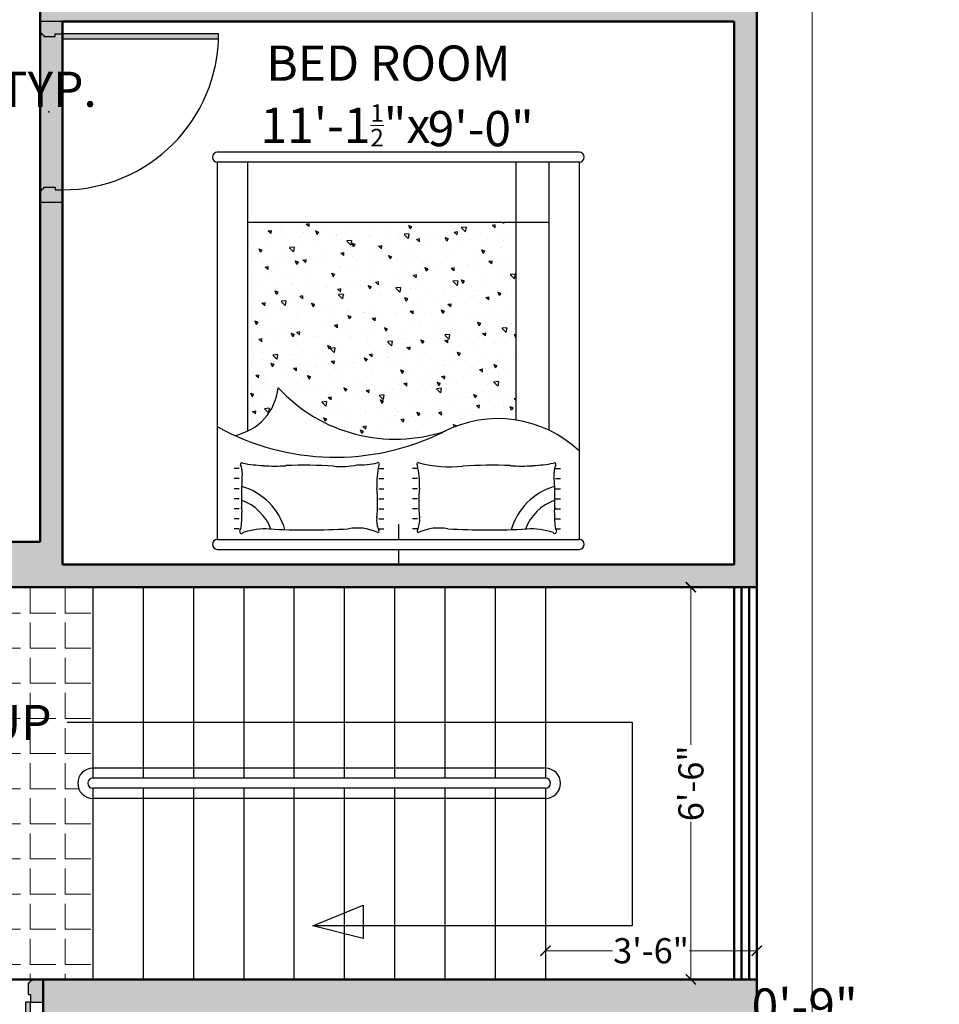
# Model space of a CAD drawing. Units: inches. Extents: x 4508 to 5907, y 877 to 1592.
# Tile 17 of 20: x 5383 to 5566, y 1298 to 1494. Entities that reach past the tile are written whole.
import ezdxf

# ---------------------------------------------------------------- set-up
doc = ezdxf.new("R2010")
doc.units = ezdxf.units.IN
doc.layers.get('DEFPOINTS').update_dxf_attribs({"color": 8})
for name, color, linetype, lineweight in [('A-ANNO-DIMS', 2, 'Continuous', 18), ('A-ANNO-TEXT', 7, 'Continuous', 25), ('A-DOOR', 4, 'Continuous', 25), ('A-FLOR-PATT', 252, 'Continuous', 13), ('A-FLOR-STRS', 5, 'Continuous', 25), ('A-FURN', 24, 'Continuous', 18), ('A-WALL', 7, 'Continuous', 50), ('A-WALL-PATT', 8, 'Continuous', 13)]:
    doc.layers.add(name, color=color, linetype=linetype, lineweight=lineweight)
doc.layers.add('doors & windows', color=30, linetype='Continuous')
doc.layers.add('furniture', color=24, linetype='Continuous')
doc.styles.get("Standard").update_dxf_attribs({"font": 'arial.ttf'})
doc.dimstyles.new('details', dxfattribs={"dimtxt": 5, "dimasz": 2, "dimexe": 2, "dimexo": 3, "dimgap": 1, "dimtad": 0, "dimdec": 1, "dimzin": 0, "dimdsep": 46, "dimlunit": 4, "dimtxsty": 'Standard', "dimblk": 'ARCHTICK', "dimcen": 3, "dimclrd": 256, "dimclre": 256, "dimclrt": 256, "dimadec": 0, "dimazin": 0, "dimtfac": 0.5, "dimtdec": 1, "dimtofl": 0, "dimtmove": 0, "dimatfit": 3, "dimldrblk": 'CLOSEDBLANK', "dimfxl": 2, "dimtolj": 1, "dimtzin": 0, "dimlwd": -1, "dimlwe": -1, "dimarcsym": 0})
doc.dimstyles.new('text', dxfattribs={"dimtxt": 7, "dimasz": 0, "dimexe": 3, "dimexo": 3, "dimgap": 0, "dimtad": 1, "dimtih": 1, "dimtoh": 1, "dimzin": 3, "dimdsep": 46, "dimlunit": 4, "dimtxsty": 'Standard', "dimblk": 'CLOSEDBLANK', "dimcen": 3, "dimse1": 1, "dimse2": 1, "dimsd1": 1, "dimsd2": 1, "dimclrd": 256, "dimclre": 256, "dimclrt": 256, "dimadec": 0, "dimazin": 0, "dimtfac": 0.5, "dimtofl": 0, "dimtmove": 0, "dimatfit": 3, "dimfxl": 3, "dimtolj": 1, "dimtzin": 0, "dimlwd": -1, "dimlwe": -1, "dimarcsym": 0})

# ---------------------------------------------------------------- blocks, each defined once
blk = doc.blocks.new('bed')
at = {"layer": 'furniture'}
h = blk.add_hatch(dxfattribs=at)
h.set_pattern_fill('AR-CONC', color=256, angle=-90, style=0)
h.set_pattern_definition([(320, (0, 2.38), (-0.6275, -7.1726), [0.75, -8.25]), (265, (0, 2.38), (7.5219, 1.3875), [0.6, -6.6]), (10.451, (-0.052, 1.782), (6.8944, -5.7851), [0.6374, -7.0114]), (316.184, (2, 2.38), (-1.6552, -10.6724), [1.125, -12.375]), (6.636, (1.862, 1.491), (9.7412, -9.3466), [0.9561, -10.5171]), (261.184, (2, 2.38), (9.7412, -9.3466), [0.9, -9.9]), (291, (1.5, 1.38), (-4.0262, -5.96907), [0.75, -8.25]), (236, (1.5, 1.38), (7.2515, -2.43315), [0.6, -6.6]), (341.451, (1.1645, 0.8826), (3.2253, -8.4022), [0.6374, -7.0114]), (307.5, (0, 2.38), (3.32894, -0.1216), [0, -6.52, 0, -6.7, 0, -6.625]), (277.5, (0, 2.38), (3.94412, -2.6307), [0, -3.82, 0, -6.37, 0, -2.525]), (237.5, (0, 4.61), (-0.22555, -5.33822), [0, -2.5, 0, -7.8, 0, -10.35]), (227.5, (0, 5.61), (1.00105, -5.83186), [0, -3.25, 0, -5.18, 0, -7.35])])
h.paths.add_polyline_path([(30.01, -68), (30.01, -26.5, 0.263043), (23.9, -35.15, 0.293424), (-9.18, -26.47, -0.156683), (-23.39, -28.72), (-23.39, -68)])
for p, q in [((0, -3), (0, 0)), ((36.01, -3), (-36.01, -3)), ((-36.01, -5), (-36.01, -80)), ((36.01, -5), (-36.01, -5)), ((0, -8), (0, -5)), ((36.01, -80), (36.01, -5)), ((-31.24, -7.07), (-32.24, -7.07)), ((-3.81, -7.07), (-2.81, -7.07)), ((3.89, -7.07), (2.89, -7.07)), ((31.63, -7.07), (32.63, -7.07)), ((-31.24, -9.07), (-32.24, -9.07)), ((-3.81, -9.07), (-2.81, -9.07)), ((3.89, -9.07), (2.89, -9.07)), ((31.63, -9.07), (32.63, -9.07)), ((-31.24, -11.07), (-32.24, -11.07)), ((-3.81, -11.07), (-2.81, -11.07)), ((3.89, -11.07), (2.89, -11.07)), ((31.63, -11.07), (32.63, -11.07)), ((-31.24, -13.07), (-32.24, -13.07)), ((-3.81, -13.07), (-2.81, -13.07)), ((3.89, -13.07), (2.89, -13.07)), ((31.63, -13.07), (32.63, -13.07)), ((-31.24, -15.07), (-32.24, -15.07)), ((-3.81, -15.07), (-2.81, -15.07)), ((3.89, -15.07), (2.89, -15.07)), ((31.63, -15.07), (32.63, -15.07)), ((-31.24, -17.07), (-32.24, -17.07)), ((-3.81, -17.07), (-2.81, -17.07)), ((3.89, -17.07), (2.89, -17.07)), ((31.63, -17.07), (32.63, -17.07)), ((-31.24, -19.07), (-32.24, -19.07)), ((-3.81, -19.07), (-2.81, -19.07)), ((3.89, -19.07), (2.89, -19.07)), ((31.63, -19.07), (32.63, -19.07)), ((-36.01, -80), (36.01, -80)), ((-36.01, -82), (36.01, -82))]:
    blk.add_line(p, q, dxfattribs=at)
at = {"layer": 'furniture', "ltscale": 5}
blk.add_line((-30.01, -26.66), (-30.01, -80), dxfattribs=at)
at = {"layer": 'furniture', "ltscale": 7}
blk.add_line((30.01, -80), (30.01, -26.5), dxfattribs=at)
at = {"layer": 'furniture', "ltscale": 0.3}
for p, q in [((-23.39, -80), (-23.39, -28.72)), ((-30.01, -68), (30.01, -68))]:
    blk.add_line(p, q, dxfattribs=at)
at = {"layer": 'furniture'}
for centre, radius, start, end in [((-35.95, -4), 1, 93.3831, 266.6169), ((35.95, -4), 1, 273.3831, 86.6169), ((-31.1, -6.57), 0.382, 35.8976, 208.6272), ((-44.44, -13.85), 14.82, 27.1629, 28.6272), ((-46.76, -9.65), 15.72, 357.4804, 9.3956), ((-34.45, -3.51), 9.85, 289.8695, 338.9843), ((-34.45, -3.51), 12.47, 286.0319, 344.1205), ((-26.35, 6.68), 13.76, 251.1782, 273.3982), ((-18.02, -163.6), 156.72, 87.0032, 92.7497), ((-8.03, 2.03), 9.29, 258.896, 294.7184), ((0.25, -8.8), 4.49, 159.0146, 186.273), ((-4.03, -6.67), 0.282, 335.7259, 114.303), ((3.22, -9.94), 7.68, 155.7259, 159.0146), ((4.11, -6.67), 0.282, 65.697, 204.2741), ((-3.14, -9.94), 7.68, 20.9854, 24.2741), ((-0.17, -8.8), 4.49, 353.727, 20.9854), ((8.12, 2.03), 9.29, 245.2816, 281.104), ((18.1, -163.6), 156.72, 87.2503, 92.9968), ((34.54, -3.51), 12.47, 195.8795, 253.9681), ((34.54, -3.51), 9.85, 201.0157, 250.1305), ((26.43, 6.68), 13.76, 266.6018, 288.8218), ((31.18, -6.57), 0.382, 331.3728, 144.1024), ((46.84, -9.65), 15.72, 170.6044, 182.5196), ((44.53, -13.85), 14.82, 151.3728, 152.8371), ((-32.82, -12.44), 28.78, 354.3784, 6.273), ((32.9, -12.44), 28.78, 173.727, 185.6216), ((-28.62, 31.03), 42.31, 266.4836, 266.6487), ((54.88, -13.16), 85.99, 178.1209, 183.3613), ((-54.8, -13.16), 85.99, 356.6387, 1.8791), ((28.7, 31.03), 42.31, 273.3513, 273.5164), ((12.28, -16.11), 16.48, 177.0317, 192.8678), ((-12.19, -16.11), 16.48, 347.1322, 2.9683), ((-33.2, -18.55), 2.25, 327.6219, 339.2246), ((-34.13, -18.41), 3.18, 342.7809, 3.755), ((-18.49, 70.49), 90.23, 267.5921, 273.6329), ((-10.31, -44.95), 25.52, 75.952, 95.5452), ((11.44, -34.81), 15.32, 84.694, 102.0355), ((18.57, 70.49), 90.23, 266.3671, 272.4079), ((34.21, -18.41), 3.18, 176.245, 197.2191), ((33.28, -18.55), 2.25, 200.7754, 212.3781), ((-31.05, -19.91), 0.291, 147.6219, 311.9343), ((-24.4, -58.01), 38.42, 93.5164, 99.6766), ((-24.52, -56.06), 36.48, 86.4836, 93.5164), ((12.51, -69.71), 48.38, 60.9345, 116.3227), ((-3.95, -19.99), 0.265, 231.9005, 52.8902), ((4.03, -19.99), 0.265, 127.1098, 308.0995), ((7.57, -34.68), 14.87, 87.3976, 103.1191), ((24.6, -56.06), 36.48, 86.4836, 93.5164), ((24.48, -58.01), 38.42, 80.3234, 86.4836), ((31.13, -19.91), 0.291, 228.0657, 32.3781), ((-19.79, -5.47), 23.53, 226.4061, 297.4441), ((0.6, -56.57), 31.65, 42.5874, 108.5034), ((34.61, -36.23), 10.76, 101.1719, 174.259), ((-35.95, -81), 1, 93.3831, 266.6169), ((35.95, -81), 1, 273.3831, 86.6169)]:
    blk.add_arc(centre, radius, start, end, dxfattribs=at)
blk = doc.blocks.new('*D82')
at = {"layer": 'DEFPOINTS', "color": 0, "transparency": 16777216}
for p in [(5255.4, 1510.81), (5387.4, 1507.41), (5387.4, 1493.7)]:
    blk.add_point(p, dxfattribs=at)
at = {"layer": 'A-ANNO-DIMS', "color": 0, "transparency": 16777216, "insert": (5317.71, 1516.81), "char_height": 7, "width": 116.2892, "attachment_point": 5}
blk.add_mtext('\\A1;       HALL\\P11\'-0"x', dxfattribs=at)
blk = doc.blocks.new('_ClosedBlank')
at = {"color": 0, "lineweight": -2}
for p, q in [((-1, 0.167), (0, 0)), ((-1, 0.167), (-1, -0.167)), ((0, 0), (-1, -0.167))]:
    blk.add_line(p, q, dxfattribs=at)
blk = doc.blocks.new('*D84')
at = {"layer": 'DEFPOINTS', "color": 0, "transparency": 16777216}
for p in [(5391.9, 1468.59), (5525.4, 1468.87), (5525.4, 1463.1)]:
    blk.add_point(p, dxfattribs=at)
at = {"layer": 'A-ANNO-DIMS', "color": 0, "transparency": 16777216, "insert": (5448.13, 1478.86), "char_height": 7, "width": 124.1748, "attachment_point": 5}
blk.add_mtext('\\A1;        BED ROOM\\P11\'-1{\\H0.5x;\\S1/2;}"x', dxfattribs=at)
blk = doc.blocks.new('*D85')
at = {"layer": 'DEFPOINTS', "color": 0, "transparency": 16777216}
for p in [(5475.03, 1493.7), (5478.91, 1493.7), (5471.69, 1385.7)]:
    blk.add_point(p, dxfattribs=at)
at = {"layer": 'A-ANNO-DIMS', "color": 0, "transparency": 16777216, "insert": (5475.03, 1472.37), "char_height": 7, "attachment_point": 5}
blk.add_mtext('\\A1;9\'-0"', dxfattribs=at)
blk = doc.blocks.new('D1')
at = {"layer": 'doors & windows'}
h = blk.add_hatch(dxfattribs=at)
h.set_pattern_fill('DOTS', color=256, scale=2, angle=180, style=0)
h.set_pattern_definition([(180, (-2e-12, -4), (-0.0625, -0.125), [0, -0.125])])
h.paths.add_polyline_path([(2.5, 0), (3.5, 0), (3.5, 30.98, 0.008066), (2.5, 31)])
h = blk.add_hatch(dxfattribs=at)
h.set_pattern_fill('DOTS', color=256, scale=2, angle=180, style=0)
h.set_pattern_definition([(180, (0, -0.5), (-0.0625, -0.125), [0, -0.125])])
h.paths.add_polyline_path([(0, -4.5), (2.25, -4.5), (2.25, -4.25, 0.403966), (2.75, -3.75), (3, -3.75), (3, -1.5), (2.5, -1.5), (2.5, 0), (0, 0)])
h.paths.add_polyline_path([(36, -4.5), (36, 0), (33.5, 0), (33.5, -1.5), (33, -1.5), (33, -3.75), (33.25, -3.75, 0.403966), (33.75, -4.25), (33.75, -4.5)])
for p, q in [((0, 0), (0, -4.5)), ((36, 0), (36, -4.5))]:
    blk.add_line(p, q)
blk.add_lwpolyline([(3.5, 0), (3.5, 31), (2.5, 31), (2.5, 0)], close=True, dxfattribs=at)
for points in [[(3, -3.75), (3, -1.5), (2.5, -1.5), (2.5, 0), (0, 0)], [(33, -3.75), (33, -1.5), (33.5, -1.5), (33.5, 0), (36, 0)], [(0, -4.5), (2.25, -4.5)], [(36, -4.5), (33.75, -4.5)]]:
    blk.add_lwpolyline(points, dxfattribs=at)
for points in [[(2.25, -4.5), (2.25, -4.25, 0.403966), (2.75, -3.75), (3, -3.75)], [(33.75, -4.5), (33.75, -4.25, -0.403966), (33.25, -3.75), (33, -3.75)]]:
    blk.add_lwpolyline(points, format="xyb", dxfattribs=at)
at = {"layer": 'doors & windows', "ltscale": 6}
blk.add_arc((2.5, 0), 31, 0, 90, dxfattribs=at)
at = {"layer": 'doors & windows'}
blk.add_point((18, -2.75), dxfattribs=at)
blk = doc.blocks.new('_ArchTick')
at = {"color": 0, "linetype": 'ByBlock', "const_width": 0.15}
blk.add_lwpolyline([(-0.5, -0.5), (0.5, 0.5)], dxfattribs=at)
blk = doc.blocks.new('*D88')
at = {"layer": 'A-ANNO-DIMS', "color": 0, "transparency": 16777216}
for p, q in [((5487.9, 1306.2), (5487.9, 1310.91)), ((5529.9, 1306.2), (5529.9, 1310.91)), ((5487.9, 1308.91), (5501.26, 1308.91)), ((5529.9, 1308.91), (5516.55, 1308.91))]:
    blk.add_line(p, q, dxfattribs=at)
at = {"layer": 'DEFPOINTS', "color": 0, "transparency": 16777216}
for p in [(5487.9, 1308.91), (5487.9, 1303.2), (5529.9, 1303.2)]:
    blk.add_point(p, dxfattribs=at)
at = {"layer": 'A-ANNO-DIMS', "color": 0, "transparency": 16777216, "xscale": 2, "yscale": 2, "zscale": 2, "rotation": 180}
blk.add_blockref('_ArchTick', (5487.9, 1308.91), dxfattribs=at)
at = {"layer": 'A-ANNO-DIMS', "color": 0, "transparency": 16777216, "xscale": 2, "yscale": 2, "zscale": 2}
blk.add_blockref('_ArchTick', (5529.9, 1308.91), dxfattribs=at)
at = {"layer": 'A-ANNO-DIMS', "color": 0, "transparency": 16777216, "insert": (5508.9, 1308.91), "char_height": 5, "attachment_point": 5}
blk.add_mtext('\\A1;3\'-6"', dxfattribs=at)
blk = doc.blocks.new('*D89')
at = {"layer": 'A-ANNO-DIMS', "color": 0, "transparency": 16777216}
for p, q in [((5526.9, 1381.2), (5514.82, 1381.2)), ((5516.82, 1381.2), (5516.82, 1349.86)), ((5516.82, 1303.2), (5516.82, 1334.54)), ((5526.9, 1303.2), (5514.82, 1303.2))]:
    blk.add_line(p, q, dxfattribs=at)
at = {"layer": 'DEFPOINTS', "color": 0, "transparency": 16777216}
for p in [(5529.9, 1381.2), (5516.82, 1303.2), (5529.9, 1303.2)]:
    blk.add_point(p, dxfattribs=at)
at = {"layer": 'A-ANNO-DIMS', "color": 0, "transparency": 16777216, "xscale": 2, "yscale": 2, "zscale": 2}
for p, rotation in [((5516.82, 1381.2), 90), ((5516.82, 1303.2), 270)]:
    blk.add_blockref('_ArchTick', p, dxfattribs=dict(at, rotation=rotation))
at = {"layer": 'A-ANNO-DIMS', "color": 0, "transparency": 16777216, "insert": (5516.82, 1342.2), "char_height": 5, "attachment_point": 5, "rotation": 90}
blk.add_mtext('\\A1;6\'-6"', dxfattribs=at)
blk = doc.blocks.new('MD')
at = {"layer": 'doors & windows'}
h = blk.add_hatch(dxfattribs=at)
h.set_pattern_fill('DOTS', color=256, scale=2, style=0)
h.set_pattern_definition([(180, (0, -4), (-0.0625, 0.125), [0, -0.125])])
h.paths.add_polyline_path([(2.5, 37), (3.5, 37), (3.5, 0), (2.5, 0)])
h = blk.add_hatch(dxfattribs=at)
h.set_pattern_fill('DOTS', color=256, scale=2, style=0)
h.set_pattern_definition([(0, (0, -0.5), (0.0625, 0.125), [0, -0.125])])
h.paths.add_polyline_path([(42, -4.5), (42, 0), (39.5, 0), (39.5, -1.5), (39, -1.5), (39, -3.75), (39.25, -3.75, 0.403966), (39.75, -4.25), (39.75, -4.5)])
h.paths.add_polyline_path([(0, -4.5), (2.25, -4.5), (2.25, -4.25, 0.403966), (2.75, -3.75), (3, -3.75), (3, -1.5), (2.5, -1.5), (2.5, 0), (0, 0)])
for p, q in [((0, 0), (0, -4.5)), ((42, 0), (42, -4.5))]:
    blk.add_line(p, q)
blk.add_line((0, -4.5), (2.25, -4.5), dxfattribs=at)
blk.add_lwpolyline([(3.5, 0), (3.5, 37), (2.5, 37), (2.5, 0)], close=True, dxfattribs=at)
for points in [[(3, -3.75), (3, -1.5), (2.5, -1.5), (2.5, 0), (0, 0)], [(39, -3.75), (39, -1.5), (39.5, -1.5), (39.5, 0), (42, 0)], [(42, -4.5), (39.75, -4.5)]]:
    blk.add_lwpolyline(points, dxfattribs=at)
for points in [[(2.25, -4.5), (2.25, -4.25, 0.403966), (2.75, -3.75), (3, -3.75)], [(39.75, -4.5), (39.75, -4.25, -0.403966), (39.25, -3.75), (39, -3.75)]]:
    blk.add_lwpolyline(points, format="xyb", dxfattribs=at)
at = {"layer": 'doors & windows', "ltscale": 6}
blk.add_arc((3.73, 1.23), 35.79, 358.0281, 91.9719, dxfattribs=at)
at = {"layer": 'doors & windows'}
blk.add_point((21, -2.75), dxfattribs=at)
blk = doc.blocks.new('*D113')
at = {"layer": 'A-ANNO-DIMS', "color": 0, "transparency": 16777216}
for p, q in [((5532.9, 1574.7), (5542.92, 1574.7)), ((5540.92, 1574.7), (5540.92, 1255.95)), ((5540.92, 926.7), (5540.92, 1245.46)), ((5532.9, 926.7), (5542.92, 926.7))]:
    blk.add_line(p, q, dxfattribs=at)
at = {"layer": 'DEFPOINTS', "color": 0, "transparency": 16777216}
for p in [(5529.9, 1574.7), (5540.92, 1574.7), (5529.9, 926.7)]:
    blk.add_point(p, dxfattribs=at)
at = {"layer": 'A-ANNO-DIMS', "color": 0, "transparency": 16777216, "xscale": 2, "yscale": 2, "zscale": 2}
for p, rotation in [((5540.92, 1574.7), 90), ((5540.92, 926.7), 270)]:
    blk.add_blockref('_ArchTick', p, dxfattribs=dict(at, rotation=rotation))
at = {"layer": 'A-ANNO-DIMS', "color": 0, "transparency": 16777216, "insert": (5540.92, 1250.7), "char_height": 5, "attachment_point": 5, "rotation": 90}
blk.add_mtext("\\A1;54'", dxfattribs=at)
blk = doc.blocks.new('*D174')
at = {"layer": 'DEFPOINTS', "color": 0, "transparency": 16777216}
for p in [(5294.35, 1476.58), (5294.35, 1472.05), (5324.54, 1472.05)]:
    blk.add_point(p, dxfattribs=at)
at = {"layer": 'A-ANNO-DIMS', "transparency": 16777216, "insert": (5362.41, 1480.2), "char_height": 7, "attachment_point": 5}
blk.add_mtext('\\A1;CHAIR 2\'-6" TYP.', dxfattribs=at)
blk = doc.blocks.new('*D191')
at = {"layer": 'DEFPOINTS', "color": 0, "transparency": 16777216}
for p in [(5539.438529, 1302.416611), (5579.745522, 1302.416611), (5579.787188, 1293.416611)]:
    blk.add_point(p, dxfattribs=at)
at = {"layer": 'A-ANNO-DIMS', "transparency": 16777216, "insert": (5539.438529, 1297.916611), "char_height": 7, "attachment_point": 5}
blk.add_mtext('\\A1;0\'-9"', dxfattribs=at)

msp = doc.modelspace()

# ---------------------------------------------------------------- hatches: boundary and pattern name
at = {"layer": 'A-FLOR-PATT'}
h = msp.add_hatch(dxfattribs=at)
h.set_pattern_fill('ANGLE', color=256)
h.set_pattern_definition([(0, (0, 0), (0, 6.985), [5.08, -1.905]), (90, (0, 0), (-6.985, 4e-16), [5.08, -1.905])])
h.paths.add_polyline_path([(5397.903, 1339.204, -1), (5397.903, 1345.204), (5397.903, 1381.204), (5387.403, 1381.204), (5322.903, 1381.204), (5322.903, 1303.204), (5397.903, 1303.204)])
h.paths.add_polyline_path([(5327.748, 1331.048), (5384.489, 1331.048), (5384.489, 1357.216), (5327.748, 1357.216)], flags=24)
h.paths.add_polyline_path([(5375.002, 1348.889), (5392.146, 1348.889), (5392.146, 1359.568), (5375.002, 1359.568)], flags=24)
at = {"layer": 'A-WALL-PATT'}
h = msp.add_hatch(color=256, dxfattribs=at)
h.dxf.hatch_style = 1
h.paths.add_polyline_path([(5529.903, 1303.204), (5388.02, 1303.204), (5388.02, 1294.204), (5391.903, 1294.204), (5391.903, 1205.704), (5396.403, 1205.704), (5396.403, 1294.204), (5489.403, 1294.204), (5489.403, 1256.139), (5493.903, 1256.139), (5493.903, 1294.204), (5529.903, 1294.204)], flags=17)
h.paths.add_polyline_path([(5346.02, 1303.204), (5322.903, 1303.204), (5322.903, 1321.388), (5313.903, 1321.388), (5313.903, 1303.204), (5259.903, 1303.204), (5259.903, 1381.204), (5313.903, 1381.204), (5313.903, 1359.674), (5322.903, 1359.674), (5322.903, 1381.204), (5338.979, 1381.204), (5338.979, 1390.204), (5331.903, 1390.204), (5331.903, 1442.704), (5255.403, 1442.704), (5255.403, 1570.204), (5387.403, 1570.204), (5387.403, 1541.271), (5391.903, 1541.271), (5391.903, 1570.204), (5483.403, 1570.204), (5483.403, 1498.204), (5391.903, 1498.204), (5391.903, 1509.559), (5387.403, 1509.559), (5387.403, 1390.204), (5380.979, 1390.204), (5380.979, 1381.204), (5387.403, 1381.204), (5529.903, 1381.204), (5529.903, 1498.204), (5487.903, 1498.204), (5487.903, 1570.204), (5529.903, 1570.204), (5529.903, 1574.704), (5250.903, 1574.704), (5250.903, 991.204), (5310.903, 991.204), (5310.903, 926.704), (5529.903, 926.704), (5529.903, 1210.204), (5525.403, 1210.204), (5525.403, 1103.704), (5499.903, 1103.704), (5499.903, 1210.204), (5493.903, 1210.204), (5493.903, 1256.139), (5489.403, 1256.139), (5489.403, 1210.204), (5461.584, 1210.204), (5461.584, 1205.704), (5495.403, 1205.704), (5495.403, 1103.704), (5436.903, 1103.704), (5436.903, 1051.204), (5391.954, 1051.204), (5391.954, 1103.03), (5391.954, 1107.53), (5255.403, 1108.204), (5255.403, 1294.204), (5346.02, 1294.204)])
h.paths.add_polyline_path([(5255.403, 1390.204), (5255.403, 1398.204), (5255.403, 1438.204), (5257.903, 1438.204), (5258.903, 1438.204), (5327.403, 1438.204), (5327.403, 1390.204), (5325.903, 1390.204)], flags=16)
h.paths.add_polyline_path([(5288.757, 1390.704), (5288.757, 1390.204), (5292.173, 1390.204), (5292.173, 1390.704)], flags=0)
h.paths.add_polyline_path([(5289.965, 1391.606), (5289.965, 1396.645), (5289.903, 1396.645), (5289.903, 1397.319), (5288.849, 1398.862), (5288.849, 1398.8), (5288.983, 1398.748), (5288.983, 1399.204), (5289.091, 1399.204), (5292.081, 1399.204), (5292.081, 1398.665), (5291.946, 1398.665), (5291.027, 1397.319), (5291.027, 1396.645), (5290.965, 1396.645), (5290.965, 1391.606)], flags=0)
h.paths.add_polyline_path([(5288.849, 1399.069, 2.6374395), (5289.056, 1398.835), (5289.117, 1399.087, 0.9346155)], flags=0)
h.paths.add_polyline_path([(5290.061, 1398.665), (5290.061, 1399.204), (5290.038, 1398.975)], flags=0)
h.paths.add_polyline_path([(5291.946, 1398.934, -1), (5291.946, 1398.665)], flags=0)
h.paths.add_polyline_path([(5289.414, 1398.967), (5289.414, 1399.204), (5289.63, 1399.204), (5289.63, 1398.363), (5290.051, 1397.184), (5290.76, 1397.184), (5290.869, 1398.665), (5290.869, 1399.204), (5290.815, 1398.665), (5290.815, 1399.204), (5291.462, 1399.204), (5291.462, 1398.816), (5290.879, 1397.184), (5290.051, 1397.184)], flags=0)
h.paths.add_polyline_path([(5273.903, 1392.056), (5269.591, 1392.056, 0.0901028), (5265.544, 1392.842), (5265.511, 1392.034, -0.3516542), (5265.903, 1391.546, -1), (5264.903, 1391.546, -0.3042165), (5265.213, 1392.008), (5265.167, 1392.84, 0.0880132), (5261.215, 1392.056), (5256.903, 1392.056), (5256.903, 1398.704, -0.4142136), (5259.403, 1401.204), (5271.403, 1401.204, -0.4142136), (5273.903, 1398.704)], flags=0)
h.paths.add_polyline_path([(5263.726, 1395.073, -1), (5267.08, 1395.073, -1)], flags=0)
h.paths.add_polyline_path([(5264.434, 1395.073, -0.695521), (5265.153, 1395.073, -1.1408699), (5265.403, 1395.585, -0.7522125), (5265.403, 1396.25, 0.3674806)], flags=0)
h.paths.add_polyline_path([(5265.153, 1394.399, -1), (5265.653, 1394.399, -1)], flags=0)
h.paths.add_polyline_path([(5265.905, 1395.077, -1), (5266.405, 1395.077, -1)], flags=0)
h.paths.add_polyline_path([(5307.994, 1403.113, -1), (5307.994, 1417.295), (5318.794, 1417.295, -0.4142136), (5319.794, 1416.295), (5320.794, 1416.295, -0.4142136), (5321.794, 1417.295), (5324.903, 1417.295, -0.4142136), (5325.903, 1416.295), (5325.903, 1404.113, -0.4142136), (5324.903, 1403.113), (5321.794, 1403.113, -0.4142136), (5320.794, 1404.113), (5319.794, 1404.113, -0.4142136), (5318.794, 1403.113)], flags=0)
h.paths.add_polyline_path([(5307.836, 1405.113, -1), (5307.836, 1415.295), (5315.591, 1415.295, -0.4142136), (5317.532, 1413.353), (5317.532, 1407.054, -0.4142136), (5315.591, 1405.113)], flags=0)
h.paths.add_polyline_path([(5312.032, 1408.204, -1), (5312.032, 1412.204), (5315.032, 1412.204, -0.4142136), (5316.032, 1411.204), (5316.032, 1409.204, -0.4142136), (5315.032, 1408.204)], flags=0)
h.paths.add_polyline_path([(5391.903, 1385.704), (5391.903, 1493.704), (5525.403, 1493.704), (5525.403, 1385.704)], flags=16)
h.paths.add_polyline_path([(5422.641, 1390.704), (5422.641, 1465.704, -0.9426302), (5422.641, 1467.704), (5494.547, 1467.704, -1), (5494.665, 1465.704), (5494.665, 1390.704, -0.9426302), (5494.665, 1388.704), (5422.759, 1388.704, -1)], flags=0)
h.paths.add_polyline_path([(5427.52, 1395.749, -0.0238564), (5427.614, 1403.949, 0.0884332), (5427.476, 1405.056, 0.0506693), (5427.273, 1405.463, -0.8716827), (5427.713, 1405.835, 0.0268855), (5431.815, 1405.361, 0.0306964), (5436.289, 1405.361, -0.0263641), (5445.798, 1405.259, 0.075811), (5450.408, 1405.53, 0.0687062), (5454.457, 1405.903, -1.0086747), (5454.781, 1405.482, 0.0692081), (5454.389, 1400.959, -0.0519468), (5454.356, 1394.996, 0.1195012), (5454.627, 1392.895, 0.0143508), (5454.796, 1392.489, -0.6962059), (5454.42, 1392.118, 0.1574808), (5448.747, 1392.794, -0.025536), (5432.749, 1392.774, 0.0920085), (5427.781, 1392.048, -0.9384848), (5427.137, 1392.455, 0.0063894), (5427.314, 1392.79, 0.0472995)], flags=0)
h.paths.add_polyline_path([(5426.125, 1411.372, 0.0617649), (5428.641, 1412.201), (5428.641, 1465.704), (5488.665, 1465.704), (5488.665, 1412.363, 0.2363822), (5467.6, 1412.052, -0.2252042)], flags=0)
h.paths.add_polyline_path([(5391.903, 1490.204), (5391.903, 1491.204), (5422.903, 1491.204), (5422.903, 1490.204)], flags=0)
h.paths.add_polyline_path([(5462.545, 1392.771, 0.1270318), (5462.866, 1394.996, -0.0519468), (5462.832, 1400.959, 0.0692081), (5462.441, 1405.482, -1.0086747), (5462.765, 1405.903, 0.0857004), (5471.424, 1405.259, -0.0263641), (5480.932, 1405.361, 0.0306964), (5485.407, 1405.361, 0.0268855), (5489.509, 1405.835, -0.8716827), (5489.949, 1405.463, 0.0506693), (5489.746, 1405.056, 0.0884332), (5489.608, 1403.949, -0.0238564), (5489.702, 1395.749, 0.0472995), (5489.908, 1392.79, 0.0063894), (5490.085, 1392.455, -0.9384848), (5489.441, 1392.048, 0.0920085), (5484.473, 1392.774, -0.025536), (5468.475, 1392.794, 0.1574808), (5462.802, 1392.118, -0.6962059), (5462.426, 1392.489, 0.0100173), (5462.546, 1392.771)], flags=0)
h.paths.add_polyline_path([(5387.454, 1103.03), (5387.454, 1100.53), (5387.454, 1099.53), (5387.454, 995.03), (5387.454, 991.204), (5391.954, 991.204), (5391.954, 1046.704), (5525.403, 1046.704), (5525.403, 931.182), (5391.954, 930.53), (5391.954, 960.53), (5387.454, 960.53), (5387.454, 930.53), (5315.403, 930.53), (5315.403, 991.204), (5323.403, 991.204), (5387.454, 991.204), (5387.454, 995.03), (5255.403, 995.704), (5255.403, 1103.704)], flags=16)
h.paths.add_polyline_path([(5379.264, 1062.889), (5379.264, 1060.156), (5385.764, 1061.889, -0.4526903), (5385.764, 1059.889), (5379.264, 1059.889), (5379.264, 1055.156), (5385.764, 1056.889, -0.4526903), (5385.764, 1054.889), (5379.264, 1054.889), (5379.264, 1050.156), (5385.764, 1051.889, -0.4526903), (5385.764, 1049.889), (5379.264, 1049.889), (5379.264, 1010.156), (5385.764, 1011.889, -0.4526903), (5385.764, 1009.889), (5379.264, 1009.889), (5379.264, 1005.156), (5385.764, 1006.889, -0.4526903), (5385.764, 1004.889), (5379.264, 1004.889), (5379.264, 1000.156), (5385.764, 1001.889, -0.4526903), (5385.764, 999.889), (5378.264, 999.889), (5370.764, 997.889, -0.6674863), (5370.764, 999.889), (5377.264, 999.889), (5377.264, 1004.623), (5370.764, 1002.889, -0.6674863), (5370.764, 1004.889), (5377.264, 1004.889), (5377.264, 1009.623), (5370.764, 1007.889, -0.6674863), (5370.764, 1009.889), (5377.264, 1009.889), (5377.264, 1049.623), (5370.764, 1047.889, -0.6674863), (5370.764, 1049.889), (5377.264, 1049.889), (5377.264, 1054.623), (5370.764, 1052.889, -0.6674863), (5370.764, 1054.889), (5377.264, 1054.889), (5377.264, 1059.623), (5370.764, 1057.889, -0.6674863), (5370.764, 1059.889), (5377.264, 1059.889), (5377.264, 1062.889)], flags=0)
h.paths.add_polyline_path([(5287.641, 1000.704), (5359.665, 1000.704), (5359.665, 1018.212, 0.3202856), (5332.6, 1022.052, -0.246494), (5287.641, 1023.128)], flags=0)
h.paths.add_polyline_path([(5359.547, 1077.704, -1), (5359.665, 1075.704), (5353.665, 1075.704), (5353.665, 1063.704), (5293.641, 1063.704), (5293.641, 1075.704), (5287.759, 1075.704, -1), (5287.641, 1077.704)], flags=0)
h.paths.add_polyline_path([(5441.403, 1099.204), (5525.403, 1099.204), (5525.403, 1051.204), (5441.403, 1051.204), (5441.403, 1059.204)], flags=16)
h.paths.add_polyline_path([(5441.403, 1096.704), (5466.403, 1096.704), (5466.403, 1095.704), (5441.403, 1095.704)], flags=0)
h.paths.add_polyline_path([(5445.403, 1062.204), (5457.403, 1062.204, -0.4142136), (5459.903, 1059.704), (5459.903, 1053.056), (5455.591, 1053.056, 0.0901028), (5451.544, 1053.842), (5451.511, 1053.034, -0.3516542), (5451.903, 1052.546, -1), (5450.903, 1052.546, -0.3042165), (5451.213, 1053.008), (5451.167, 1053.84, 0.0880132), (5447.215, 1053.056), (5442.903, 1053.056), (5442.903, 1059.704, -0.4142136)], flags=0)
h.paths.add_polyline_path([(5453.08, 1056.073, -1), (5449.726, 1056.073, -1)], flags=0)
h.paths.add_polyline_path([(5292.713, 1015.835, 0.0268855), (5296.815, 1015.361, 0.0306964), (5301.289, 1015.361, -0.0263641), (5310.798, 1015.259, 0.075811), (5315.408, 1015.53, 0.0687062), (5319.457, 1015.903, -1.0086747), (5319.781, 1015.482, 0.0692081), (5319.389, 1010.959, -0.0519468), (5319.356, 1004.996, 0.1195012), (5319.627, 1002.895, 0.0143508), (5319.796, 1002.489, -0.6962059), (5319.42, 1002.118, 0.1574808), (5313.747, 1002.794, -0.025536), (5297.749, 1002.774, 0.0920085), (5292.781, 1002.048, -0.9384848), (5292.137, 1002.455, 0.0063894), (5292.314, 1002.79, 0.0472995), (5292.52, 1005.749, -0.0238564), (5292.614, 1013.949, 0.0884332), (5292.476, 1015.056, 0.0506693), (5292.273, 1015.463, -0.8716827)], flags=0)
h.paths.add_polyline_path([(5450.434, 1056.073, -0.695521), (5451.153, 1056.073, -1.1408699), (5451.403, 1056.585, -0.7522125), (5451.403, 1057.25, 0.3674806)], flags=0)
h.paths.add_polyline_path([(5327.765, 1015.903, 0.0857004), (5336.424, 1015.259, -0.0263641), (5345.932, 1015.361, 0.0306964), (5350.407, 1015.361, 0.0268855), (5354.509, 1015.835, -0.8716827), (5354.949, 1015.463, 0.0506693), (5354.746, 1015.056, 0.0884332), (5354.608, 1013.949, -0.0238564), (5354.702, 1005.749, 0.0472995), (5354.908, 1002.79, 0.0063894), (5355.085, 1002.455, -0.9384848), (5354.441, 1002.048, 0.0920085), (5349.473, 1002.774, -0.025536), (5333.475, 1002.794, 0.1574808), (5327.802, 1002.118, -0.6962059), (5327.426, 1002.489, 0.0100173), (5327.546, 1002.771), (5327.545, 1002.771, 0.1270318), (5327.866, 1004.996, -0.0519468), (5327.832, 1010.959, 0.0692081), (5327.441, 1015.482, -1.0086747)], flags=0)
h.paths.add_polyline_path([(5452.405, 1056.077, -1), (5451.905, 1056.077, -1)], flags=0)
h.paths.add_polyline_path([(5451.653, 1055.399, -1), (5451.153, 1055.399, -1)], flags=0)
h.paths.add_polyline_path([(5472.958, 1051.704), (5472.958, 1051.204), (5476.374, 1051.204), (5476.374, 1051.704)], flags=0)
h.paths.add_polyline_path([(5476.282, 1060.204), (5476.282, 1059.665), (5476.147, 1059.665), (5475.228, 1058.319), (5475.228, 1057.645), (5475.166, 1052.606), (5474.166, 1052.606), (5474.166, 1057.645), (5474.104, 1057.645), (5474.104, 1058.319), (5473.05, 1059.862), (5473.05, 1059.8), (5473.184, 1059.748), (5473.184, 1060.204), (5473.292, 1060.204)], flags=0)
h.paths.add_polyline_path([(5473.05, 1060.069, 2.6374395), (5473.257, 1059.835), (5473.318, 1060.087, 0.9346155)], flags=0)
h.paths.add_polyline_path([(5473.831, 1060.204), (5473.831, 1059.363), (5474.252, 1058.184), (5474.371, 1058.184), (5474.262, 1059.665), (5474.262, 1060.204)], flags=0)
h.paths.add_polyline_path([(5475.501, 1060.204), (5475.501, 1059.363), (5475.555, 1059.514), (5475.555, 1060.204)], flags=0)
h.paths.add_polyline_path([(5474.855, 1060.204), (5474.908, 1060.127), (5474.908, 1060.204), (5474.855, 1059.665)], flags=0)
h.paths.add_polyline_path([(5476.147, 1059.934, -1), (5476.147, 1059.665)], flags=0)
h.paths.add_polyline_path([(5474.693, 1060.204), (5475.178, 1059.511), (5475.178, 1060.204), (5475.285, 1059.934), (5475.285, 1060.204), (5475.178, 1059.665), (5475.178, 1060.204), (5475.07, 1059.665), (5475.07, 1060.204), (5474.962, 1059.665), (5474.962, 1060.204), (5474.693, 1059.306)], flags=0)
h.paths.add_polyline_path([(5474.747, 1060.204), (5474.37, 1059.45), (5474.37, 1060.204), (5474.424, 1060.096), (5474.424, 1060.204), (5474.747, 1059.665)], flags=0)
h.paths.add_polyline_path([(5476.04, 1059.665), (5476.04, 1060.204), (5476.094, 1059.665), (5476.094, 1060.204)], flags=0)
h.paths.add_polyline_path([(5505.994, 1082.295), (5516.794, 1082.295, -0.4142136), (5517.794, 1081.295), (5518.794, 1081.295, -0.4142136), (5519.794, 1082.295), (5522.903, 1082.295, -0.4142136), (5523.903, 1081.295), (5523.903, 1069.113, -0.4142136), (5522.903, 1068.113), (5519.794, 1068.113, -0.4142136), (5518.794, 1069.113), (5517.794, 1069.113, -0.4142136), (5516.794, 1068.113), (5505.994, 1068.113, -1)], flags=0)
h.paths.add_polyline_path([(5505.836, 1080.295), (5513.591, 1080.295, -0.4142136), (5515.532, 1078.353), (5515.532, 1072.054, -0.4142136), (5513.591, 1070.113), (5505.836, 1070.113, -1)], flags=0)
h.paths.add_polyline_path([(5520.403, 963.695), (5520.403, 1035.72), (5502.895, 1035.72, 0.3202856), (5499.055, 1008.654, -0.246494), (5497.978, 963.695)], flags=0)
h.paths.add_polyline_path([(5445.403, 1035.72), (5445.403, 1029.72), (5457.403, 1029.72), (5457.403, 969.695), (5445.403, 969.695), (5445.403, 963.814, -1), (5443.403, 963.695), (5443.403, 1035.602, -1)], flags=0)
h.paths.add_polyline_path([(5510.032, 1077.204), (5513.032, 1077.204, -0.4142136), (5514.032, 1076.204), (5514.032, 1074.204, -0.4142136), (5513.032, 1073.204), (5510.032, 1073.204, -1)], flags=0)
h.paths.add_polyline_path([(5317.255, 989.704), (5323.903, 989.704, -0.4142136), (5326.403, 987.204), (5326.403, 975.204, -0.4142136), (5323.903, 972.704), (5317.255, 972.704), (5317.255, 977.016, 0.0901028), (5318.041, 981.063), (5317.233, 981.096, -0.8964437), (5316.245, 981.204, -0.8220123), (5317.207, 981.394), (5318.04, 981.44, 0.0880132), (5317.255, 985.392)], flags=0)
h.paths.add_polyline_path([(5321.949, 981.204, -1), (5318.594, 981.204, -1)], flags=0)
h.paths.add_polyline_path([(5362.454, 988.03), (5387.454, 988.03), (5387.454, 990.53), (5391.954, 990.53), (5391.704, 988.289, -0.4090807), (5391.204, 987.78), (5391.204, 987.53), (5388.954, 987.53), (5388.954, 988.03), (5387.454, 988.03), (5387.454, 987.03), (5362.474, 987.03, 0.4025427), (5387.454, 963.03), (5388.954, 963.03), (5388.954, 963.53), (5391.195, 963.28, -0.4142136), (5391.704, 962.771), (5391.954, 960.53), (5391.954, 962.78), (5391.704, 962.78, 0.4090807), (5391.195, 963.28), (5388.954, 963.53), (5388.954, 963.03), (5387.454, 963.03, -0.4025427), (5362.474, 987.03), (5362.454, 987.03)], flags=0)
h.paths.add_polyline_path([(5321.285, 981.204, -0.6555366), (5320.522, 981.204, -1.1195284), (5320.275, 980.701, -1.3500746), (5320.279, 980.026, 0.3749463)], flags=0)
h.paths.add_polyline_path([(5320.022, 981.923, -1), (5320.522, 981.923, -1)], flags=0)
h.paths.add_polyline_path([(5319.348, 981.204, -1), (5319.848, 981.204, -1)], flags=0)
h.paths.add_polyline_path([(5507.157, 1030.662, -0.0238564), (5515.358, 1030.756, 0.0472995), (5518.317, 1030.962, 0.0063894), (5518.652, 1031.139, -0.9384848), (5519.059, 1030.495, 0.0920085), (5518.333, 1025.527, -0.025536), (5518.313, 1009.53, 0.1574808), (5518.989, 1003.857, -0.6962059), (5518.618, 1003.48, 0.0100173), (5518.335, 1003.601), (5518.335, 1003.6, 0.1270318), (5516.111, 1003.921, -0.0519468), (5510.148, 1003.887, 0.0692081), (5505.624, 1003.495, -1.0086747), (5505.204, 1003.819, 0.0857004), (5505.848, 1012.479, -0.0263641), (5505.746, 1021.987, 0.0306964), (5505.746, 1026.462, 0.0268855), (5505.272, 1030.563, -0.8716827), (5505.644, 1031.004, 0.0506693), (5506.051, 1030.801, 0.0884332)], flags=0)
h.paths.add_polyline_path([(5368.045, 945.621), (5378.845, 945.621, -0.4142136), (5379.845, 944.621), (5380.845, 944.621, -0.4142136), (5381.845, 945.621), (5384.954, 945.621, -0.4142136), (5385.954, 944.621), (5385.954, 932.439, -0.4142136), (5384.954, 931.439), (5381.845, 931.439, -0.4142136), (5380.845, 932.439), (5379.845, 932.439, -0.4142136), (5378.845, 931.439), (5368.045, 931.439, -1)], flags=0)
h.paths.add_polyline_path([(5327.31, 931.03), (5327.31, 930.53), (5330.726, 930.53), (5330.726, 931.03)], flags=0)
h.paths.add_polyline_path([(5330.634, 939.53), (5330.634, 938.991), (5330.499, 938.991), (5329.579, 937.645), (5329.579, 936.971), (5329.518, 936.971), (5329.518, 931.933), (5328.518, 931.933), (5328.518, 936.971), (5328.456, 936.971), (5328.456, 937.645), (5327.402, 939.189), (5327.402, 939.126), (5327.536, 939.074), (5327.536, 939.53), (5327.644, 939.53)], flags=0)
h.paths.add_polyline_path([(5327.402, 939.395, 2.6374395), (5327.609, 939.161), (5327.67, 939.414, 0.9346155)], flags=0)
h.paths.add_polyline_path([(5328.021, 939.142), (5328.021, 939.53), (5327.967, 939.53), (5327.967, 939.293)], flags=0)
h.paths.add_polyline_path([(5328.614, 939.53), (5328.614, 938.991), (5328.723, 937.51), (5329.313, 937.51), (5329.422, 938.991), (5329.422, 939.53), (5329.368, 938.991), (5329.368, 939.53)], flags=0)
h.paths.add_polyline_path([(5329.853, 939.53), (5329.853, 938.689), (5329.907, 938.84), (5329.907, 939.53)], flags=0)
h.paths.add_polyline_path([(5330.499, 939.261, -1), (5330.499, 938.991)], flags=0)
h.paths.add_polyline_path([(5367.887, 943.621), (5375.641, 943.621, -0.4142136), (5377.583, 941.68), (5377.583, 935.38, -0.4142136), (5375.641, 933.439), (5367.887, 933.439, -1)], flags=0)
h.paths.add_polyline_path([(5509.267, 947.14), (5509.267, 939.64), (5511.267, 932.14, -0.4526903), (5509.267, 932.14), (5509.267, 938.64), (5504.534, 938.64), (5506.267, 932.14, -0.4526903), (5504.267, 932.14), (5504.267, 938.64), (5499.534, 938.64), (5501.267, 932.14, -0.4526903), (5499.267, 932.14), (5499.267, 938.64), (5459.534, 938.64), (5461.267, 932.14, -0.4526903), (5459.267, 932.14), (5459.267, 938.64), (5454.534, 938.64), (5456.267, 932.14, -0.4526903), (5454.267, 932.14), (5454.267, 938.64), (5449.534, 938.64), (5451.267, 932.14, -0.4526903), (5449.267, 932.14), (5449.267, 939.64), (5447.267, 947.14, -0.3030853), (5448.267, 947.808), (5508.266, 947.808, -0.3032033)], flags=0)
h.paths.add_polyline_path([(5510.148, 995.444, -0.0519468), (5516.111, 995.41, 0.1195012), (5518.212, 995.681, 0.0143508), (5518.618, 995.851, -0.6962059), (5518.989, 995.474, 0.1574808), (5518.313, 989.801, -0.025536), (5518.333, 973.804, 0.0920085), (5519.059, 968.836, -0.9384848), (5518.652, 968.192, 0.0063894), (5518.317, 968.369, 0.0472995), (5515.358, 968.575, -0.0238564), (5507.157, 968.669, 0.0884332), (5506.051, 968.531, 0.0506693), (5505.644, 968.327, -0.8716827), (5505.272, 968.768, 0.0268855), (5505.746, 972.869, 0.0306964), (5505.746, 977.344, -0.0263641), (5505.848, 986.852, 0.075811), (5505.576, 991.462, 0.0687062), (5505.204, 995.512, -1.0086747), (5505.624, 995.836, 0.0692081)], flags=0)
h.paths.add_polyline_path([(5372.083, 940.53), (5375.083, 940.53, -0.4142136), (5376.083, 939.53), (5376.083, 937.53, -0.4142136), (5375.083, 936.53), (5372.083, 936.53, -1)], flags=0)
h.paths.add_polyline_path([(5409.258, 1465.643), (5487.738, 1465.643), (5487.738, 1492.394), (5409.258, 1492.394)], flags=8)
h.paths.add_polyline_path([(5463.574, 1465.103), (5486.546, 1465.103), (5486.546, 1479.528), (5463.574, 1479.528)], flags=8)
h.paths.add_polyline_path([(5248.665, 1406.171), (5299.981, 1406.171), (5299.981, 1432.34), (5248.665, 1432.34)], flags=9)
h.paths.add_polyline_path([(5287.471, 1405.121), (5310.443, 1405.121), (5310.443, 1419.546), (5287.471, 1419.546)], flags=8)
h.paths.add_polyline_path([(5371.637, 1047.927), (5371.637, 1010.764), (5377.841, 1010.764), (5377.841, 1047.927)], flags=8)
h.paths.add_polyline_path([(5324.882, 1074.869), (5347.854, 1074.869), (5347.854, 1089.294), (5324.882, 1089.294)], flags=8)
h.paths.add_polyline_path([(5262.863, 1074.665), (5351.123, 1074.665), (5351.123, 1100.833), (5262.863, 1100.833)], flags=8)
h.paths.add_polyline_path([(5307.238, 938.814), (5363.988, 938.814), (5363.988, 964.982), (5307.238, 964.982)], flags=24)
h.paths.add_polyline_path([(5348.837, 937.997), (5371.809, 937.997), (5371.809, 952.422), (5348.837, 952.422)], flags=8)
h.paths.add_polyline_path([(5432.497, 1066.695), (5489.247, 1066.695), (5489.247, 1092.863), (5432.497, 1092.863)], flags=24)
h.paths.add_polyline_path([(5473.52, 1065.943), (5496.492, 1065.943), (5496.492, 1080.368), (5473.52, 1080.368)], flags=8)
h.paths.add_polyline_path([(5451.783, 984.266), (5480.194, 984.266), (5480.194, 998.691), (5451.783, 998.691)], flags=8)
h.paths.add_polyline_path([(5392.211, 983.632), (5481.554, 983.632), (5481.554, 1010.383), (5392.211, 1010.383)], flags=8)
h.paths.add_polyline_path([(5497.304, 946.267), (5460.142, 946.267), (5460.142, 940.062), (5497.304, 940.062)], flags=8)

# ---------------------------------------------------------------- linework, layer by layer
at = {"layer": 'A-FLOR-STRS'}
for p, q in [((5397.903, 1381.204), (5397.903, 1343.204)), ((5407.903, 1381.204), (5407.903, 1343.204)), ((5417.903, 1381.204), (5417.903, 1343.204)), ((5427.903, 1381.204), (5427.903, 1343.204)), ((5437.903, 1381.204), (5437.903, 1343.204)), ((5447.903, 1381.204), (5447.903, 1343.204)), ((5457.903, 1381.204), (5457.903, 1343.204)), ((5467.903, 1381.204), (5467.903, 1343.204)), ((5477.903, 1381.204), (5477.903, 1343.204)), ((5487.903, 1381.204), (5487.903, 1343.204)), ((5487.903, 1345.204), (5397.903, 1345.204)), ((5487.903, 1343.204), (5397.903, 1343.204)), ((5487.903, 1341.204), (5397.903, 1341.204)), ((5397.903, 1341.204), (5397.903, 1303.204)), ((5407.903, 1341.204), (5407.903, 1303.204)), ((5417.903, 1341.204), (5417.903, 1303.204)), ((5427.903, 1341.204), (5427.903, 1303.204)), ((5437.903, 1341.204), (5437.903, 1303.204)), ((5447.903, 1341.204), (5447.903, 1303.204)), ((5457.903, 1341.204), (5457.903, 1303.204)), ((5467.903, 1341.204), (5467.903, 1303.204)), ((5477.903, 1341.204), (5477.903, 1303.204)), ((5487.903, 1341.204), (5487.903, 1303.204)), ((5487.903, 1339.204), (5397.903, 1339.204))]:
    msp.add_line(p, q, dxfattribs=at)
msp.add_lwpolyline([(5392.797, 1354.37), (5505.126, 1354.37), (5505.126, 1313.87), (5441.63, 1313.87), (5451.63, 1317.999), (5451.63, 1311.322), (5441.63, 1313.87)], dxfattribs=at)
for centre, radius, start, end in [((5397.903, 1342.204), 3, 90, 270), ((5487.903, 1342.204), 3, 270, 90), ((5397.903, 1342.204), 1, 90, 270), ((5487.903, 1342.204), 1, 270, 90)]:
    msp.add_arc(centre, radius, start, end, dxfattribs=at)
at = {"layer": 'A-WALL'}
for p, q in [((5529.903, 1574.704), (5529.903, 926.704)), ((5387.403, 1509.559), (5387.403, 1390.204)), ((5391.903, 1493.704), (5525.403, 1493.704)), ((5391.903, 1493.704), (5391.903, 1385.704)), ((5525.403, 1493.704), (5525.403, 1385.704)), ((5331.903, 1390.204), (5387.403, 1390.204)), ((5391.903, 1385.704), (5525.403, 1385.704)), ((5322.903, 1381.204), (5387.403, 1381.204)), ((5387.403, 1381.204), (5529.903, 1381.204)), ((5525.403, 1381.204), (5525.403, 1303.204)), ((5526.903, 1381.204), (5526.903, 1303.204)), ((5528.403, 1381.204), (5528.403, 1303.204)), ((5322.903, 1303.204), (5529.903, 1303.204)), ((5388.02, 1303.204), (5388.02, 1294.204))]:
    msp.add_line(p, q, dxfattribs=at)

# ---------------------------------------------------------------- block references
at = {"layer": 'A-DOOR'}
for name, p, rotation in [('D1', (5391.903, 1493.704), 270), ('MD', (5388.02, 1298.704), 180)]:
    msp.add_blockref(name, p, dxfattribs=dict(at, rotation=rotation))
at = {"layer": 'A-FURN', "rotation": 180}
msp.add_blockref('bed', (5458.653, 1385.704), dxfattribs=at)

# ---------------------------------------------------------------- texts
at = {"layer": 'A-ANNO-TEXT'}
msp.add_text('UP', height=7, dxfattribs=at).set_placement((5376.782, 1350.788))

# ---------------------------------------------------------------- dimensions: what is measured, and where the dimension line sits
at = {"layer": 'A-ANNO-DIMS'}
for base, p1, p2, dimstyle, override, picture, middle in [((5540.921, 1574.704), (5529.903, 926.704), (5529.903, 1574.704), 'details', {"dimclrd": 0, "dimclre": 0, "dimclrt": 0}, '*D113', (5540.921, 1250.704)), ((5516.825, 1303.204), (5529.903, 1381.204), (5529.903, 1303.204), 'details', {"dimclrd": 0, "dimclre": 0, "dimclrt": 0}, '*D89', (5516.825, 1342.204)), ((5539.439, 1302.417), (5579.787, 1293.417), (5579.746, 1302.417), 'text', {"dimdec": 1, "dimlfac": 1, "dimrnd": 0, "dimzin": 1, "dimdsep": 46, "dimlunit": 4, "dimfrac": 2}, '*D191', (5539.439, 1297.917))]:
    dim = msp.add_linear_dim(base=base, p1=p1, p2=p2, angle=90, dimstyle=dimstyle, override=override, dxfattribs=at)
    dim.commit()
    dim.dimension.update_dxf_attribs({"geometry": picture, "text_midpoint": middle})
for base, p1, p2, text, picture, middle in [((5387.403, 1507.406), (5255.403, 1510.807), (5387.403, 1493.704), '       HALL\\P<>x', '*D82', (5317.713, 1507.406)), ((5525.403, 1468.867), (5391.903, 1468.588), (5525.403, 1463.097), '        BED ROOM\\P<>x', '*D84', (5448.128, 1468.867))]:
    dim = msp.add_linear_dim(base=base, p1=p1, p2=p2, text=text, dimstyle='text', override={"dimclrd": 0, "dimclre": 0, "dimclrt": 0}, dxfattribs=at)
    dim.commit()
    dim.dimension.update_dxf_attribs({"geometry": picture, "text_midpoint": middle, "dimtype": 160})
dim = msp.add_linear_dim(base=(5294.351, 1476.577), p1=(5324.541, 1472.048), p2=(5294.351, 1472.048), angle=180, text='CHAIR <> TYP.', dimstyle='text', override={"dimdec": 1, "dimrnd": 0, "dimzin": 1, "dimlunit": 4, "dimfrac": 2}, dxfattribs=at)
dim.commit()
dim.dimension.update_dxf_attribs({"geometry": '*D174', "text_midpoint": (5362.406, 1480.196)})
dim = msp.add_linear_dim(base=(5475.034, 1493.704), p1=(5471.693, 1385.704), p2=(5478.907, 1493.704), angle=90, dimstyle='text', override={"dimtad": 0, "dimclrd": 0, "dimclre": 0, "dimclrt": 0}, dxfattribs=at)
dim.commit()
dim.dimension.update_dxf_attribs({"geometry": '*D85', "text_midpoint": (5475.034, 1472.365), "dimtype": 160})
dim = msp.add_linear_dim(base=(5487.903, 1308.908), p1=(5529.903, 1303.204), p2=(5487.903, 1303.204), dimstyle='details', override={"dimclrd": 0, "dimclre": 0, "dimclrt": 0}, dxfattribs=at)
dim.commit()
dim.dimension.update_dxf_attribs({"geometry": '*D88', "text_midpoint": (5508.903, 1308.908)})

doc.saveas('drawing.dxf')
